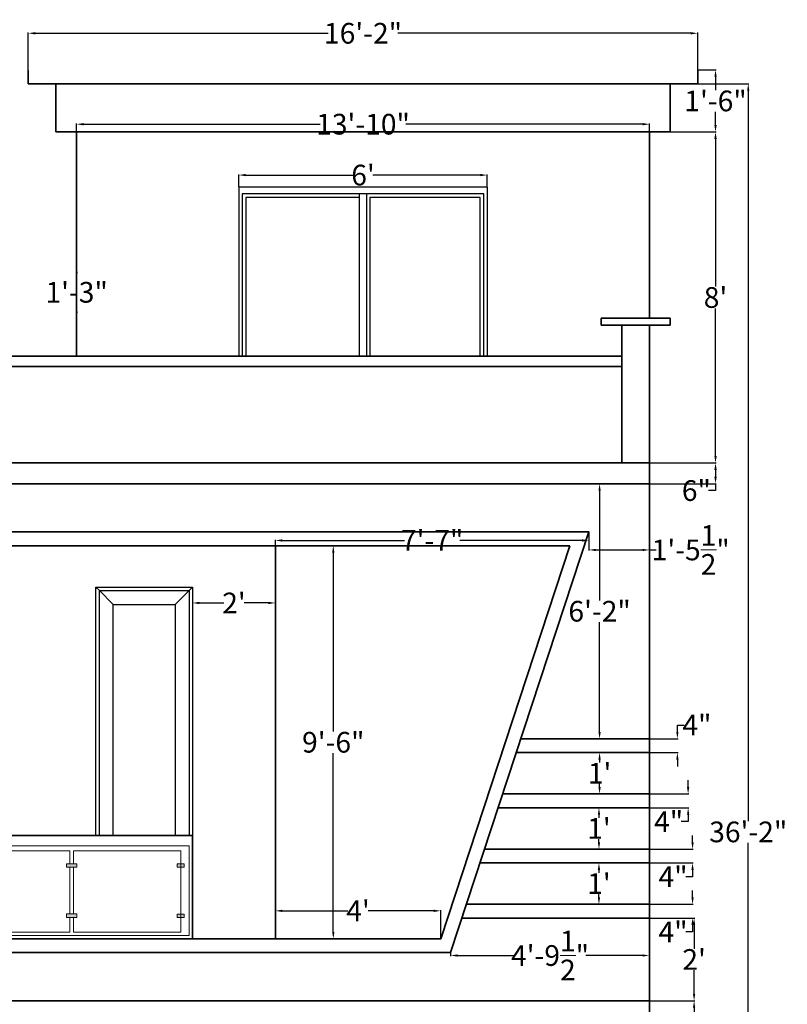
# Model space of a CAD drawing. Units: inches. Extents: x 786 to 1239, y 110 to 563.
# Tile 3 of 3: x 1017 to 1239, y 277 to 563. Entities that reach past the tile are written whole.
import ezdxf

# ---------------------------------------------------------------- set-up
doc = ezdxf.new("R2010")
doc.units = ezdxf.units.IN
doc.header["$MEASUREMENT"] = 0
for name, color, linetype, lineweight in [('A-ANNO-DIMS', 2, 'Continuous', 18), ('A-ELEV', 7, 'Continuous', 35), ('A-ELEV-PATT', 8, 'Continuous', 13), ('A-ELEV-RAIL', 3, 'Continuous', 18), ('A-GLAZ', 4, 'Continuous', 25)]:
    doc.layers.add(name, color=color, linetype=linetype, lineweight=lineweight)
doc.styles.get("Standard").update_dxf_attribs({"font": 'arial.ttf'})
doc.dimstyles.get("Standard").update_dxf_attribs({"dimtxt": 6, "dimasz": 2, "dimexe": 0.18, "dimexo": 0.0625, "dimgap": 0.09, "dimtad": 0, "dimtih": 1, "dimtoh": 1, "dimdec": 1, "dimzin": 0, "dimdsep": 46, "dimlunit": 4, "dimtxsty": 'Standard', "dimcen": 0.09, "dimadec": 0, "dimazin": 0, "dimtfac": 1, "dimtdec": 1, "dimtofl": 0, "dimtmove": 0, "dimatfit": 3, "dimfxl": 1, "dimtolj": 1, "dimtzin": 0, "dimarcsym": 0})

# ---------------------------------------------------------------- blocks, each defined once
blk = doc.blocks.new('*D10')
at = {"layer": 'A-ANNO-DIMS', "color": 0, "lineweight": -2, "transparency": 16777216}
for p, q in [((1199.19, 428.05), (1199.19, 408.71)), ((1181.65, 414.05), (1181.65, 408.71)), ((1183.65, 408.89), (1197.19, 408.89)), ((1199.19, 408.89), (1201.19, 408.89))]:
    blk.add_line(p, q, dxfattribs=at)
at = {"layer": 'A-ANNO-DIMS', "color": 0, "transparency": 16777216}
for points in [[(1183.65, 409.22), (1183.65, 408.56), (1181.65, 408.89)], [(1197.19, 409.22), (1197.19, 408.56), (1199.19, 408.89)]]:
    blk.add_solid(points, dxfattribs=at)
at = {"layer": 'Defpoints', "color": 0, "transparency": 16777216}
for p in [(1199.19, 428.11), (1181.65, 414.11), (1199.19, 408.89)]:
    blk.add_point(p, dxfattribs=at)
at = {"layer": 'A-ANNO-DIMS', "color": 0, "transparency": 16777216, "insert": (1211.16, 408.89), "char_height": 6, "attachment_point": 5}
blk.add_mtext('\\A1;1\'-5{\\H1x;\\S1/2;}"', dxfattribs=at)
blk = doc.blocks.new('*D11')
at = {"layer": 'A-ANNO-DIMS', "color": 0, "lineweight": -2, "transparency": 16777216}
for p, q in [((1090.86, 410.11), (1107.75, 410.11)), ((1107.57, 408.11), (1107.57, 356.26)), ((1107.57, 298.11), (1107.57, 349.96)), ((1090.86, 296.11), (1107.75, 296.11))]:
    blk.add_line(p, q, dxfattribs=at)
at = {"layer": 'A-ANNO-DIMS', "color": 0, "transparency": 16777216}
for points in [[(1107.24, 408.11), (1107.91, 408.11), (1107.57, 410.11)], [(1107.24, 298.11), (1107.91, 298.11), (1107.57, 296.11)]]:
    blk.add_solid(points, dxfattribs=at)
at = {"layer": 'Defpoints', "color": 0, "transparency": 16777216}
for p in [(1090.79, 410.11), (1107.57, 410.11), (1090.79, 296.11)]:
    blk.add_point(p, dxfattribs=at)
at = {"layer": 'A-ANNO-DIMS', "color": 0, "transparency": 16777216, "insert": (1107.57, 353.11), "char_height": 6, "attachment_point": 5}
blk.add_mtext('\\A1;9\'-6"', dxfattribs=at)
blk = doc.blocks.new('*D14')
at = {"layer": 'A-ANNO-DIMS', "color": 0, "lineweight": -2, "transparency": 16777216}
for p, q in [((1033.19, 489.11), (1033.19, 486.76)), ((1033.26, 491.11), (1033.37, 491.11)), ((1033.19, 478.11), (1033.19, 480.45)), ((1033.26, 476.11), (1033.37, 476.11))]:
    blk.add_line(p, q, dxfattribs=at)
at = {"layer": 'A-ANNO-DIMS', "color": 0, "transparency": 16777216}
for points in [[(1032.86, 489.11), (1033.53, 489.11), (1033.19, 491.11)], [(1032.86, 478.11), (1033.53, 478.11), (1033.19, 476.11)]]:
    blk.add_solid(points, dxfattribs=at)
at = {"layer": 'Defpoints', "color": 0, "transparency": 16777216}
for p in [(1033.19, 491.11), (1033.19, 491.11), (1033.19, 476.11)]:
    blk.add_point(p, dxfattribs=at)
at = {"layer": 'A-ANNO-DIMS', "color": 0, "transparency": 16777216, "insert": (1033.19, 483.61), "char_height": 6, "attachment_point": 5}
blk.add_mtext('\\A1;1\'-3"', dxfattribs=at)
blk = doc.blocks.new('*D15')
at = {"layer": 'A-ANNO-DIMS', "color": 0, "lineweight": -2, "transparency": 16777216}
for p, q in [((1080.19, 514.19), (1080.19, 517.79)), ((1082.19, 517.61), (1113.33, 517.61)), ((1150.19, 517.61), (1119.06, 517.61)), ((1152.19, 514.19), (1152.19, 517.79))]:
    blk.add_line(p, q, dxfattribs=at)
at = {"layer": 'A-ANNO-DIMS', "color": 0, "transparency": 16777216}
for points in [[(1082.19, 517.95), (1082.19, 517.28), (1080.19, 517.61)], [(1150.19, 517.95), (1150.19, 517.28), (1152.19, 517.61)]]:
    blk.add_solid(points, dxfattribs=at)
at = {"layer": 'Defpoints', "color": 0, "transparency": 16777216}
for p in [(1080.19, 517.61), (1080.19, 514.13), (1152.19, 514.13)]:
    blk.add_point(p, dxfattribs=at)
at = {"layer": 'A-ANNO-DIMS', "color": 0, "transparency": 16777216, "insert": (1116.19, 517.61), "char_height": 6, "attachment_point": 5}
blk.add_mtext("\\A1;6'", dxfattribs=at)
blk = doc.blocks.new('*D16')
at = {"layer": 'A-ANNO-DIMS', "color": 0, "lineweight": -2, "transparency": 16777216}
for p, q in [((1213.26, 548.11), (1218.53, 548.11)), ((1218.35, 546.11), (1218.35, 542.26)), ((1218.35, 532.11), (1218.35, 535.96)), ((1205.26, 530.11), (1218.53, 530.11))]:
    blk.add_line(p, q, dxfattribs=at)
at = {"layer": 'A-ANNO-DIMS', "color": 0, "transparency": 16777216}
for points in [[(1218.02, 546.11), (1218.69, 546.11), (1218.35, 548.11)], [(1218.02, 532.11), (1218.69, 532.11), (1218.35, 530.11)]]:
    blk.add_solid(points, dxfattribs=at)
at = {"layer": 'Defpoints', "color": 0, "transparency": 16777216}
for p in [(1213.19, 548.11), (1218.35, 548.11), (1205.19, 530.11)]:
    blk.add_point(p, dxfattribs=at)
at = {"layer": 'A-ANNO-DIMS', "color": 0, "transparency": 16777216, "insert": (1218.35, 539.11), "char_height": 6, "attachment_point": 5}
blk.add_mtext('\\A1;1\'-6"', dxfattribs=at)
blk = doc.blocks.new('*D17')
at = {"layer": 'A-ANNO-DIMS', "color": 0, "lineweight": -2, "transparency": 16777216}
for p, q in [((1019.19, 544.17), (1019.19, 558.92)), ((1021.19, 558.74), (1106.08, 558.74)), ((1211.19, 558.74), (1126.31, 558.74)), ((1213.19, 544.17), (1213.19, 558.92))]:
    blk.add_line(p, q, dxfattribs=at)
at = {"layer": 'A-ANNO-DIMS', "color": 0, "transparency": 16777216}
for points in [[(1021.19, 559.07), (1021.19, 558.41), (1019.19, 558.74)], [(1211.19, 559.07), (1211.19, 558.41), (1213.19, 558.74)]]:
    blk.add_solid(points, dxfattribs=at)
at = {"layer": 'Defpoints', "color": 0, "transparency": 16777216}
for p in [(1019.19, 558.74), (1019.19, 544.11), (1213.19, 544.11)]:
    blk.add_point(p, dxfattribs=at)
at = {"layer": 'A-ANNO-DIMS', "color": 0, "transparency": 16777216, "insert": (1116.19, 558.74), "char_height": 6, "attachment_point": 5}
blk.add_mtext('\\A1;16\'-2"', dxfattribs=at)
blk = doc.blocks.new('*D18')
at = {"layer": 'A-ANNO-DIMS', "color": 0, "lineweight": -2, "transparency": 16777216}
for p, q in [((1033.19, 530.17), (1033.19, 532.55)), ((1035.19, 532.37), (1103.75, 532.37)), ((1197.19, 532.37), (1128.64, 532.37)), ((1199.19, 530.17), (1199.19, 532.55))]:
    blk.add_line(p, q, dxfattribs=at)
at = {"layer": 'A-ANNO-DIMS', "color": 0, "transparency": 16777216}
for points in [[(1035.19, 532.7), (1035.19, 532.03), (1033.19, 532.37)], [(1197.19, 532.7), (1197.19, 532.03), (1199.19, 532.37)]]:
    blk.add_solid(points, dxfattribs=at)
at = {"layer": 'Defpoints', "color": 0, "transparency": 16777216}
for p in [(1199.19, 532.37), (1033.19, 530.11), (1199.19, 530.11)]:
    blk.add_point(p, dxfattribs=at)
at = {"layer": 'A-ANNO-DIMS', "color": 0, "transparency": 16777216, "insert": (1116.19, 532.37), "char_height": 6, "attachment_point": 5}
blk.add_mtext('\\A1;13\'-10"', dxfattribs=at)
blk = doc.blocks.new('*D19')
at = {"layer": 'A-ANNO-DIMS', "color": 0, "lineweight": -2, "transparency": 16777216}
for p, q in [((1207.3, 356.11), (1207.3, 358.11)), ((1207.3, 358.11), (1209.3, 358.11)), ((1199.26, 354.11), (1207.48, 354.11)), ((1199.26, 350.11), (1207.48, 350.11)), ((1207.3, 348.11), (1207.3, 346.11))]:
    blk.add_line(p, q, dxfattribs=at)
at = {"layer": 'A-ANNO-DIMS', "color": 0, "transparency": 16777216}
for points in [[(1206.97, 356.11), (1207.63, 356.11), (1207.3, 354.11)], [(1206.97, 348.11), (1207.63, 348.11), (1207.3, 350.11)]]:
    blk.add_solid(points, dxfattribs=at)
at = {"layer": 'Defpoints', "color": 0, "transparency": 16777216}
for p in [(1199.19, 354.11), (1207.3, 354.11), (1199.19, 350.11)]:
    blk.add_point(p, dxfattribs=at)
at = {"layer": 'A-ANNO-DIMS', "color": 0, "transparency": 16777216, "insert": (1212.96, 358.11), "char_height": 6, "attachment_point": 5}
blk.add_mtext('\\A1;4"', dxfattribs=at)
blk = doc.blocks.new('*D20')
at = {"layer": 'A-ANNO-DIMS', "color": 0, "lineweight": -2, "transparency": 16777216}
for p, q in [((1210.41, 340.11), (1210.41, 342.11)), ((1199.26, 338.11), (1210.59, 338.11)), ((1199.26, 334.11), (1210.59, 334.11)), ((1210.41, 332.11), (1210.41, 330.11)), ((1210.41, 330.11), (1208.41, 330.11))]:
    blk.add_line(p, q, dxfattribs=at)
at = {"layer": 'A-ANNO-DIMS', "color": 0, "transparency": 16777216}
for points in [[(1210.08, 340.11), (1210.75, 340.11), (1210.41, 338.11)], [(1210.08, 332.11), (1210.75, 332.11), (1210.41, 334.11)]]:
    blk.add_solid(points, dxfattribs=at)
at = {"layer": 'Defpoints', "color": 0, "transparency": 16777216}
for p in [(1199.19, 338.11), (1199.19, 334.11), (1210.41, 334.11)]:
    blk.add_point(p, dxfattribs=at)
at = {"layer": 'A-ANNO-DIMS', "color": 0, "transparency": 16777216, "insert": (1204.76, 330.11), "char_height": 6, "attachment_point": 5}
blk.add_mtext('\\A1;4"', dxfattribs=at)
blk = doc.blocks.new('*D21')
at = {"layer": 'A-ANNO-DIMS', "color": 0, "lineweight": -2, "transparency": 16777216}
for p, q in [((1211.7, 324.11), (1211.7, 326.11)), ((1199.26, 322.11), (1211.88, 322.11)), ((1199.26, 318.11), (1211.88, 318.11)), ((1211.7, 316.11), (1211.7, 314.11)), ((1211.7, 314.11), (1209.7, 314.11))]:
    blk.add_line(p, q, dxfattribs=at)
at = {"layer": 'A-ANNO-DIMS', "color": 0, "transparency": 16777216}
for points in [[(1211.37, 324.11), (1212.03, 324.11), (1211.7, 322.11)], [(1211.37, 316.11), (1212.03, 316.11), (1211.7, 318.11)]]:
    blk.add_solid(points, dxfattribs=at)
at = {"layer": 'Defpoints', "color": 0, "transparency": 16777216}
for p in [(1199.19, 322.11), (1199.19, 318.11), (1211.7, 318.11)]:
    blk.add_point(p, dxfattribs=at)
at = {"layer": 'A-ANNO-DIMS', "color": 0, "transparency": 16777216, "insert": (1206.04, 314.11), "char_height": 6, "attachment_point": 5}
blk.add_mtext('\\A1;4"', dxfattribs=at)
blk = doc.blocks.new('*D22')
at = {"layer": 'A-ANNO-DIMS', "color": 0, "lineweight": -2, "transparency": 16777216}
for p, q in [((1211.7, 308.11), (1211.7, 310.11)), ((1199.26, 306.11), (1211.88, 306.11)), ((1199.26, 302.11), (1211.88, 302.11)), ((1211.7, 300.11), (1211.7, 298.11)), ((1211.7, 298.11), (1209.7, 298.11))]:
    blk.add_line(p, q, dxfattribs=at)
at = {"layer": 'A-ANNO-DIMS', "color": 0, "transparency": 16777216}
for points in [[(1211.37, 308.11), (1212.03, 308.11), (1211.7, 306.11)], [(1211.37, 300.11), (1212.03, 300.11), (1211.7, 302.11)]]:
    blk.add_solid(points, dxfattribs=at)
at = {"layer": 'Defpoints', "color": 0, "transparency": 16777216}
for p in [(1199.19, 306.11), (1199.19, 302.11), (1211.7, 302.11)]:
    blk.add_point(p, dxfattribs=at)
at = {"layer": 'A-ANNO-DIMS', "color": 0, "transparency": 16777216, "insert": (1206.04, 298.11), "char_height": 6, "attachment_point": 5}
blk.add_mtext('\\A1;4"', dxfattribs=at)
blk = doc.blocks.new('*D23')
at = {"layer": 'A-ANNO-DIMS', "color": 0, "lineweight": -2, "transparency": 16777216}
for p, q in [((1199.13, 350.11), (1184.57, 350.11)), ((1184.75, 348.11), (1184.75, 347.21)), ((1184.75, 340.11), (1184.75, 341.01)), ((1199.13, 338.11), (1184.57, 338.11))]:
    blk.add_line(p, q, dxfattribs=at)
at = {"layer": 'A-ANNO-DIMS', "color": 0, "transparency": 16777216}
for points in [[(1184.42, 348.11), (1185.08, 348.11), (1184.75, 350.11)], [(1184.42, 340.11), (1185.08, 340.11), (1184.75, 338.11)]]:
    blk.add_solid(points, dxfattribs=at)
at = {"layer": 'Defpoints', "color": 0, "transparency": 16777216}
for p in [(1199.19, 350.11), (1184.75, 338.11), (1199.19, 338.11)]:
    blk.add_point(p, dxfattribs=at)
at = {"layer": 'A-ANNO-DIMS', "color": 0, "transparency": 16777216, "insert": (1184.75, 344.11), "char_height": 6, "attachment_point": 5}
blk.add_mtext("\\A1;1'", dxfattribs=at)
blk = doc.blocks.new('*D36')
at = {"layer": 'A-ANNO-DIMS', "color": 0, "lineweight": -2, "transparency": 16777216}
for p, q in [((1199.26, 278.11), (1212.32, 278.11)), ((1212.14, 276.11), (1212.14, 274.11)), ((1199.26, 272.11), (1212.32, 272.11)), ((1212.14, 272.11), (1212.14, 270.11)), ((1212.14, 270.11), (1210.14, 270.11))]:
    blk.add_line(p, q, dxfattribs=at)
at = {"layer": 'A-ANNO-DIMS', "color": 0, "transparency": 16777216}
for points in [[(1211.81, 276.11), (1212.47, 276.11), (1212.14, 278.11)], [(1211.81, 274.11), (1212.47, 274.11), (1212.14, 272.11)]]:
    blk.add_solid(points, dxfattribs=at)
at = {"layer": 'Defpoints', "color": 0, "transparency": 16777216}
for p in [(1199.19, 278.11), (1199.19, 272.11), (1212.14, 272.11)]:
    blk.add_point(p, dxfattribs=at)
at = {"layer": 'A-ANNO-DIMS', "color": 0, "transparency": 16777216, "insert": (1206.58, 270.11), "char_height": 6, "attachment_point": 5}
blk.add_mtext('\\A1;6"', dxfattribs=at)
blk = doc.blocks.new('*D37')
at = {"layer": 'A-ANNO-DIMS', "color": 0, "lineweight": -2, "transparency": 16777216}
for p, q in [((1199.26, 302.11), (1212.32, 302.11)), ((1212.14, 300.11), (1212.14, 293.21)), ((1212.14, 280.11), (1212.14, 287.01)), ((1199.26, 278.11), (1212.32, 278.11))]:
    blk.add_line(p, q, dxfattribs=at)
at = {"layer": 'A-ANNO-DIMS', "color": 0, "transparency": 16777216}
for points in [[(1211.81, 300.11), (1212.47, 300.11), (1212.14, 302.11)], [(1211.81, 280.11), (1212.47, 280.11), (1212.14, 278.11)]]:
    blk.add_solid(points, dxfattribs=at)
at = {"layer": 'Defpoints', "color": 0, "transparency": 16777216}
for p in [(1199.19, 302.11), (1212.14, 302.11), (1199.19, 278.11)]:
    blk.add_point(p, dxfattribs=at)
at = {"layer": 'A-ANNO-DIMS', "color": 0, "transparency": 16777216, "insert": (1212.14, 290.11), "char_height": 6, "attachment_point": 5}
blk.add_mtext("\\A1;2'", dxfattribs=at)
blk = doc.blocks.new('*D38')
at = {"layer": 'A-ANNO-DIMS', "color": 0, "lineweight": -2, "transparency": 16777216}
for p, q in [((1141.59, 292.05), (1141.59, 291.08)), ((1199.19, 278.17), (1199.19, 291.44)), ((1143.59, 291.26), (1160.02, 291.26)), ((1197.19, 291.26), (1180.77, 291.26))]:
    blk.add_line(p, q, dxfattribs=at)
at = {"layer": 'A-ANNO-DIMS', "color": 0, "transparency": 16777216}
for points in [[(1143.59, 291.59), (1143.59, 290.93), (1141.59, 291.26)], [(1197.19, 291.59), (1197.19, 290.93), (1199.19, 291.26)]]:
    blk.add_solid(points, dxfattribs=at)
at = {"layer": 'Defpoints', "color": 0, "transparency": 16777216}
for p in [(1141.59, 292.11), (1199.19, 291.26), (1199.19, 278.11)]:
    blk.add_point(p, dxfattribs=at)
at = {"layer": 'A-ANNO-DIMS', "color": 0, "transparency": 16777216, "insert": (1170.39, 291.26), "char_height": 6, "attachment_point": 5}
blk.add_mtext('\\A1;4\'-9{\\H1x;\\S1/2;}"', dxfattribs=at)
blk = doc.blocks.new('*D39')
at = {"layer": 'A-ANNO-DIMS', "color": 0, "lineweight": -2, "transparency": 16777216}
for p, q in [((1199.26, 530.11), (1218.53, 530.11)), ((1218.35, 528.11), (1218.35, 485.26)), ((1218.35, 436.11), (1218.35, 478.96)), ((1199.26, 434.11), (1218.53, 434.11))]:
    blk.add_line(p, q, dxfattribs=at)
at = {"layer": 'A-ANNO-DIMS', "color": 0, "transparency": 16777216}
for points in [[(1218.02, 528.11), (1218.69, 528.11), (1218.35, 530.11)], [(1218.02, 436.11), (1218.69, 436.11), (1218.35, 434.11)]]:
    blk.add_solid(points, dxfattribs=at)
at = {"layer": 'Defpoints', "color": 0, "transparency": 16777216}
for p in [(1199.19, 530.11), (1218.35, 530.11), (1199.19, 434.11)]:
    blk.add_point(p, dxfattribs=at)
at = {"layer": 'A-ANNO-DIMS', "color": 0, "transparency": 16777216, "insert": (1218.35, 482.11), "char_height": 6, "attachment_point": 5}
blk.add_mtext("\\A1;8'", dxfattribs=at)
blk = doc.blocks.new('*D40')
at = {"layer": 'A-ANNO-DIMS', "color": 0, "lineweight": -2, "transparency": 16777216}
for p, q in [((1199.26, 434.11), (1218.53, 434.11)), ((1218.35, 432.11), (1218.35, 430.11)), ((1199.26, 428.11), (1218.53, 428.11)), ((1218.35, 426.11), (1216.35, 426.11)), ((1218.35, 428.11), (1218.35, 426.11))]:
    blk.add_line(p, q, dxfattribs=at)
at = {"layer": 'A-ANNO-DIMS', "color": 0, "transparency": 16777216}
for points in [[(1218.02, 432.11), (1218.69, 432.11), (1218.35, 434.11)], [(1218.02, 430.11), (1218.69, 430.11), (1218.35, 428.11)]]:
    blk.add_solid(points, dxfattribs=at)
at = {"layer": 'Defpoints', "color": 0, "transparency": 16777216}
for p in [(1199.19, 434.11), (1199.19, 428.11), (1218.35, 428.11)]:
    blk.add_point(p, dxfattribs=at)
at = {"layer": 'A-ANNO-DIMS', "color": 0, "transparency": 16777216, "insert": (1212.8, 426.11), "char_height": 6, "attachment_point": 5}
blk.add_mtext('\\A1;6"', dxfattribs=at)
blk = doc.blocks.new('*D48')
at = {"layer": 'A-ANNO-DIMS', "color": 0, "lineweight": -2, "transparency": 16777216}
for p, q in [((1205.26, 544.11), (1228.02, 544.11)), ((1227.84, 542.11), (1227.84, 330.26)), ((1227.84, 112.11), (1227.84, 323.95)), ((1199.26, 110.11), (1228.02, 110.11))]:
    blk.add_line(p, q, dxfattribs=at)
at = {"layer": 'A-ANNO-DIMS', "color": 0, "transparency": 16777216}
for points in [[(1227.51, 542.11), (1228.17, 542.11), (1227.84, 544.11)], [(1227.51, 112.11), (1228.17, 112.11), (1227.84, 110.11)]]:
    blk.add_solid(points, dxfattribs=at)
at = {"layer": 'Defpoints', "color": 0, "transparency": 16777216}
for p in [(1205.19, 544.11), (1199.19, 110.11), (1227.84, 110.11)]:
    blk.add_point(p, dxfattribs=at)
at = {"layer": 'A-ANNO-DIMS', "color": 0, "transparency": 16777216, "insert": (1227.84, 327.11), "char_height": 6, "attachment_point": 5}
blk.add_mtext('\\A1;36\'-2"', dxfattribs=at)
blk = doc.blocks.new('*D49')
at = {"layer": 'A-ANNO-DIMS', "color": 0, "lineweight": -2, "transparency": 16777216}
for p, q in [((1090.79, 410.17), (1090.79, 411.83)), ((1092.79, 411.65), (1128.18, 411.65)), ((1179.65, 411.65), (1144.26, 411.65)), ((1181.65, 414.05), (1181.65, 411.47))]:
    blk.add_line(p, q, dxfattribs=at)
at = {"layer": 'A-ANNO-DIMS', "color": 0, "transparency": 16777216}
for points in [[(1092.79, 411.98), (1092.79, 411.31), (1090.79, 411.65)], [(1179.65, 411.98), (1179.65, 411.31), (1181.65, 411.65)]]:
    blk.add_solid(points, dxfattribs=at)
at = {"layer": 'Defpoints', "color": 0, "transparency": 16777216}
for p in [(1181.65, 414.11), (1181.65, 411.65), (1090.79, 410.11)]:
    blk.add_point(p, dxfattribs=at)
at = {"layer": 'A-ANNO-DIMS', "color": 0, "transparency": 16777216, "insert": (1136.22, 411.65), "char_height": 6, "attachment_point": 5}
blk.add_mtext('\\A1;7\'-7"', dxfattribs=at)
blk = doc.blocks.new('*D50')
at = {"layer": 'A-ANNO-DIMS', "color": 0, "lineweight": -2, "transparency": 16777216}
for p, q in [((1090.79, 296.17), (1090.79, 304.4)), ((1092.79, 304.22), (1111.77, 304.22)), ((1136.7, 304.22), (1117.72, 304.22)), ((1138.7, 296.17), (1138.7, 304.4))]:
    blk.add_line(p, q, dxfattribs=at)
at = {"layer": 'A-ANNO-DIMS', "color": 0, "transparency": 16777216}
for points in [[(1092.79, 304.55), (1092.79, 303.89), (1090.79, 304.22)], [(1136.7, 304.55), (1136.7, 303.89), (1138.7, 304.22)]]:
    blk.add_solid(points, dxfattribs=at)
at = {"layer": 'Defpoints', "color": 0, "transparency": 16777216}
for p in [(1090.79, 304.22), (1090.79, 296.11), (1138.7, 296.11)]:
    blk.add_point(p, dxfattribs=at)
at = {"layer": 'A-ANNO-DIMS', "color": 0, "transparency": 16777216, "insert": (1114.74, 304.22), "char_height": 6, "attachment_point": 5}
blk.add_mtext("\\A1;4'", dxfattribs=at)
blk = doc.blocks.new('*D55')
at = {"layer": 'A-ANNO-DIMS', "color": 0, "lineweight": -2, "transparency": 16777216}
for p, q in [((1090.79, 410.05), (1090.79, 393.33)), ((1066.79, 398.05), (1066.79, 393.33)), ((1068.79, 393.51), (1075.89, 393.51)), ((1088.79, 393.51), (1081.7, 393.51))]:
    blk.add_line(p, q, dxfattribs=at)
at = {"layer": 'A-ANNO-DIMS', "color": 0, "transparency": 16777216}
for points in [[(1068.79, 393.84), (1068.79, 393.18), (1066.79, 393.51)], [(1088.79, 393.84), (1088.79, 393.18), (1090.79, 393.51)]]:
    blk.add_solid(points, dxfattribs=at)
at = {"layer": 'Defpoints', "color": 0, "transparency": 16777216}
for p in [(1090.79, 410.11), (1066.79, 398.11), (1066.79, 393.51)]:
    blk.add_point(p, dxfattribs=at)
at = {"layer": 'A-ANNO-DIMS', "color": 0, "transparency": 16777216, "insert": (1078.79, 393.51), "char_height": 6, "attachment_point": 5}
blk.add_mtext("\\A1;2'", dxfattribs=at)
blk = doc.blocks.new('*D56')
at = {"layer": 'A-ANNO-DIMS', "color": 0, "lineweight": -2, "transparency": 16777216}
for p, q in [((1199.13, 334.11), (1184.39, 334.11)), ((1184.57, 332.11), (1184.57, 331.21)), ((1184.57, 324.11), (1184.57, 325.01)), ((1199.13, 322.11), (1184.39, 322.11))]:
    blk.add_line(p, q, dxfattribs=at)
at = {"layer": 'A-ANNO-DIMS', "color": 0, "transparency": 16777216}
for points in [[(1184.24, 332.11), (1184.9, 332.11), (1184.57, 334.11)], [(1184.24, 324.11), (1184.9, 324.11), (1184.57, 322.11)]]:
    blk.add_solid(points, dxfattribs=at)
at = {"layer": 'Defpoints', "color": 0, "transparency": 16777216}
for p in [(1199.19, 334.11), (1184.57, 322.11), (1199.19, 322.11)]:
    blk.add_point(p, dxfattribs=at)
at = {"layer": 'A-ANNO-DIMS', "color": 0, "transparency": 16777216, "insert": (1184.57, 328.11), "char_height": 6, "attachment_point": 5}
blk.add_mtext("\\A1;1'", dxfattribs=at)
blk = doc.blocks.new('*D57')
at = {"layer": 'A-ANNO-DIMS', "color": 0, "lineweight": -2, "transparency": 16777216}
for p, q in [((1199.13, 318.11), (1184.39, 318.11)), ((1184.57, 316.11), (1184.57, 315.21)), ((1184.57, 308.11), (1184.57, 309.01)), ((1199.13, 306.11), (1184.39, 306.11))]:
    blk.add_line(p, q, dxfattribs=at)
at = {"layer": 'A-ANNO-DIMS', "color": 0, "transparency": 16777216}
for points in [[(1184.24, 316.11), (1184.9, 316.11), (1184.57, 318.11)], [(1184.24, 308.11), (1184.9, 308.11), (1184.57, 306.11)]]:
    blk.add_solid(points, dxfattribs=at)
at = {"layer": 'Defpoints', "color": 0, "transparency": 16777216}
for p in [(1199.19, 318.11), (1184.57, 306.11), (1199.19, 306.11)]:
    blk.add_point(p, dxfattribs=at)
at = {"layer": 'A-ANNO-DIMS', "color": 0, "transparency": 16777216, "insert": (1184.57, 312.11), "char_height": 6, "attachment_point": 5}
blk.add_mtext("\\A1;1'", dxfattribs=at)
blk = doc.blocks.new('*D58')
at = {"layer": 'A-ANNO-DIMS', "color": 0, "lineweight": -2, "transparency": 16777216}
for p, q in [((1199.13, 428.11), (1184.57, 428.11)), ((1184.75, 426.11), (1184.75, 394.26)), ((1184.75, 356.11), (1184.75, 387.96)), ((1199.13, 354.11), (1184.57, 354.11))]:
    blk.add_line(p, q, dxfattribs=at)
at = {"layer": 'A-ANNO-DIMS', "color": 0, "transparency": 16777216}
for points in [[(1184.42, 426.11), (1185.08, 426.11), (1184.75, 428.11)], [(1184.42, 356.11), (1185.08, 356.11), (1184.75, 354.11)]]:
    blk.add_solid(points, dxfattribs=at)
at = {"layer": 'Defpoints', "color": 0, "transparency": 16777216}
for p in [(1184.75, 428.11), (1199.19, 428.11), (1199.19, 354.11)]:
    blk.add_point(p, dxfattribs=at)
at = {"layer": 'A-ANNO-DIMS', "color": 0, "transparency": 16777216, "insert": (1184.75, 391.11), "char_height": 6, "attachment_point": 5}
blk.add_mtext('\\A1;6\'-2"', dxfattribs=at)
blk = doc.blocks.new('GLASS-CLAMP-A')
for p, q in [((0, 1), (3, 1)), ((0, 1), (0, 0)), ((3, 0), (3, 1)), ((3, 0), (0, 0))]:
    blk.add_line(p, q)
blk = doc.blocks.new('GLASS-CLAMP-B')
for p, q in [((0, 1), (2, 1)), ((0, 0), (0, 1)), ((2, 0), (2, 1)), ((0, 0), (2, 0))]:
    blk.add_line(p, q)

msp = doc.modelspace()

# ---------------------------------------------------------------- hatches: boundary and pattern name
at = {"layer": 'A-ELEV-PATT'}
h = msp.add_hatch(color=256, dxfattribs=at)
h.dxf.hatch_style = 1
h.paths.add_polyline_path([(842.59, 317.86), (841.59, 317.86), (841.59, 316.86), (842.59, 316.86)])
h.paths.add_polyline_path([(841.59, 317.86), (840.59, 317.86), (840.59, 316.86), (841.59, 316.86)])
h.paths.add_polyline_path([(842.59, 303.29), (841.59, 303.29), (841.59, 302.31), (842.59, 302.31)])
h.paths.add_polyline_path([(841.59, 303.29), (840.59, 303.29), (840.59, 302.31), (841.59, 302.31)])
h.paths.add_polyline_path([(1064.36, 317.86), (1063.36, 317.86), (1063.36, 316.86), (1064.36, 316.86)])
h.paths.add_polyline_path([(1063.36, 317.86), (1062.36, 317.86), (1062.36, 316.86), (1063.36, 316.86)])
h.paths.add_polyline_path([(1064.36, 303.29), (1063.36, 303.29), (1063.36, 302.31), (1064.36, 302.31)])
h.paths.add_polyline_path([(1063.36, 303.29), (1062.36, 303.29), (1062.36, 302.31), (1063.36, 302.31)])
h = msp.add_hatch(color=256, dxfattribs=at)
h.dxf.hatch_style = 1
h.paths.add_polyline_path([(874.65, 317.86), (871.65, 317.86), (871.65, 316.86), (874.65, 316.86)])
h.paths.add_polyline_path([(906.56, 317.86), (903.56, 317.86), (903.56, 316.86), (906.56, 316.86)])
h.paths.add_polyline_path([(938.2, 317.86), (935.2, 317.86), (935.2, 316.86), (938.2, 316.86)])
h.paths.add_polyline_path([(969.78, 317.86), (966.78, 317.86), (966.78, 316.86), (969.78, 316.86)])
h.paths.add_polyline_path([(1001.46, 317.86), (998.46, 317.86), (998.46, 316.86), (1001.46, 316.86)])
h.paths.add_polyline_path([(1033.24, 317.86), (1030.24, 317.86), (1030.24, 316.86), (1033.24, 316.86)])
h.paths.add_polyline_path([(1033.24, 303.31), (1030.24, 303.31), (1030.24, 302.31), (1033.24, 302.31)])
h.paths.add_polyline_path([(1001.46, 303.31), (998.46, 303.31), (998.46, 302.31), (1001.46, 302.31)])
h.paths.add_polyline_path([(969.78, 303.31), (966.78, 303.31), (966.78, 302.31), (969.78, 302.31)])
h.paths.add_polyline_path([(938.2, 303.31), (935.2, 303.31), (935.2, 302.31), (938.2, 302.31)])
h.paths.add_polyline_path([(906.56, 303.31), (903.56, 303.31), (903.56, 302.31), (906.56, 302.31)])
h.paths.add_polyline_path([(874.65, 303.31), (871.65, 303.31), (871.65, 302.31), (874.65, 302.31)])

# ---------------------------------------------------------------- linework, layer by layer
at = {"layer": 'A-ELEV'}
for p, q in [((1019.19, 547.93), (1019.19, 544.11)), ((1213.19, 544.11), (1213.19, 548.11)), ((1213.19, 544.11), (1019.19, 544.11)), ((1027.19, 530.11), (1027.19, 544.11)), ((1205.19, 530.11), (1205.19, 544.11)), ((1205.19, 530.11), (1027.19, 530.11)), ((1033.19, 465.11), (1033.19, 530.11)), ((1199.19, 530.11), (1199.19, 476.11)), ((1205.19, 476.11), (1185.19, 476.11)), ((1185.19, 474.11), (1185.19, 476.11)), ((1199.19, 474.11), (1185.19, 474.11)), ((1191.19, 434.11), (1191.19, 474.11)), ((1199.19, 434.11), (1199.19, 474.11)), ((1199.19, 474.11), (1205.19, 474.11)), ((1205.19, 474.11), (1205.19, 476.11)), ((1191.19, 465.11), (983.67, 465.11)), ((1191.19, 462.11), (983.67, 462.11)), ((1191.19, 434.11), (815.19, 434.11)), ((1199.19, 434.11), (1191.19, 434.11)), ((1199.19, 428.11), (1199.19, 434.11)), ((1199.19, 428.11), (815.19, 428.11)), ((1199.19, 410.11), (1199.19, 428.11)), ((1176.13, 410.11), (839.19, 410.11)), ((1090.79, 296.11), (1090.79, 410.11)), ((1176.13, 410.11), (1138.7, 296.11)), ((1199.19, 278.11), (1199.19, 410.11)), ((1199.19, 354.11), (1161.95, 354.11)), ((1160.64, 350.11), (1199.19, 350.11)), ((1199.19, 338.11), (1156.7, 338.11)), ((1155.38, 334.11), (1199.19, 334.11)), ((1066.79, 326.11), (839.19, 326.11)), ((1066.79, 326.11), (1066.79, 296.11)), ((1199.19, 322.11), (1151.44, 322.11)), ((1150.13, 318.11), (1199.19, 318.11)), ((1199.19, 306.11), (1146.19, 306.11)), ((1144.88, 302.11), (1199.19, 302.11)), ((1138.7, 296.11), (839.19, 296.11)), ((1199.19, 278.11), (815.19, 278.11)), ((1199.19, 272.11), (1199.19, 278.11))]:
    msp.add_line(p, q, dxfattribs=at)
msp.add_lwpolyline([(1141.59, 292.11), (835.19, 292.11), (835.19, 414.11), (1181.65, 414.11)], close=True, dxfattribs=at)
at = {"layer": 'A-ELEV-RAIL'}
for p, q in [((1065.79, 323.11), (840.19, 323.11)), ((1065.79, 297.11), (1065.79, 323.11)), ((1065.79, 297.11), (840.19, 297.11))]:
    msp.add_line(p, q, dxfattribs=at)
for points in [[(1000.18, 317.86), (1000.18, 321.66), (1031.24, 321.66), (1031.24, 317.86)], [(1032.31, 317.86), (1032.31, 321.66), (1063.36, 321.66), (1063.36, 298.05), (1032.31, 298.05), (1032.31, 302.31)], [(1031.24, 316.86), (1031.24, 303.31)], [(1032.31, 303.31), (1032.31, 316.86)], [(1031.24, 302.31), (1031.24, 298.05), (1000.18, 298.05), (1000.18, 302.31)]]:
    msp.add_lwpolyline(points, dxfattribs=at)
at = {"layer": 'A-GLAZ'}
for p, q in [((1080.19, 514.13), (1080.19, 465.11)), ((1152.19, 514.13), (1080.19, 514.13)), ((1152.19, 514.13), (1152.19, 465.11)), ((1115.19, 465.11), (1115.19, 512.13)), ((1117.19, 512.13), (1117.19, 465.11)), ((1118.19, 511.13), (1118.19, 465.11)), ((1039.79, 397.11), (1038.79, 398.11)), ((1043.79, 393.11), (1039.79, 397.11)), ((1061.79, 393.11), (1065.79, 397.11)), ((1065.79, 397.11), (1066.79, 398.11))]:
    msp.add_line(p, q, dxfattribs=at)
for points in [[(1151.19, 465.11), (1151.19, 512.13), (1081.19, 512.13), (1081.19, 465.11)], [(1115.19, 511.13), (1082.19, 511.13), (1082.19, 465.11)], [(1150.19, 465.11), (1150.19, 511.13), (1118.19, 511.13)], [(1038.79, 326.11), (1038.79, 398.11), (1066.79, 398.11), (1066.79, 326.11)], [(1039.79, 326.11), (1039.79, 397.11), (1065.79, 397.11), (1065.79, 326.11)], [(1043.79, 326.11), (1043.79, 393.11), (1061.79, 393.11), (1061.79, 326.11)]]:
    msp.add_lwpolyline(points, dxfattribs=at)

# ---------------------------------------------------------------- block references
at = {"layer": 'A-ELEV-RAIL'}
for name, p, rotation in [('GLASS-CLAMP-A', (1033.24, 317.86), 180), ('GLASS-CLAMP-B', (1064.36, 317.86), 180), ('GLASS-CLAMP-A', (1033.24, 303.31), 180), ('GLASS-CLAMP-B', (1062.36, 302.3), 359.7010863405159)]:
    msp.add_blockref(name, p, dxfattribs=dict(at, rotation=rotation))

# ---------------------------------------------------------------- dimensions: what is measured, and where the dimension line sits
at = {"layer": 'A-ANNO-DIMS'}
for base, p1, p2, picture, middle in [((1019.19, 558.74), (1213.19, 544.11), (1019.19, 544.11), '*D17', (1116.19, 558.74)), ((1199.19, 532.37), (1033.19, 530.11), (1199.19, 530.11), '*D18', (1116.19, 532.37)), ((1080.19, 517.61), (1152.19, 514.13), (1080.19, 514.13), '*D15', (1116.19, 517.61)), ((1199.19, 408.89), (1181.65, 414.11), (1199.19, 428.11), '*D10', (1211.16, 408.89)), ((1181.65, 411.65), (1090.79, 410.11), (1181.65, 414.11), '*D49', (1136.22, 411.65)), ((1066.79, 393.51), (1090.79, 410.11), (1066.79, 398.11), '*D55', (1078.79, 393.51)), ((1090.79, 304.22), (1138.7, 296.11), (1090.79, 296.11), '*D50', (1114.74, 304.22)), ((1199.19, 291.26), (1141.59, 292.11), (1199.19, 278.11), '*D38', (1170.39, 291.26))]:
    dim = msp.add_linear_dim(base=base, p1=p1, p2=p2, dimstyle='Standard', override={"dimclrd": 0, "dimclre": 0, "dimclrt": 0}, dxfattribs=at)
    dim.commit()
    dim.dimension.update_dxf_attribs({"geometry": picture, "text_midpoint": middle})
for base, p1, p2, picture, middle in [((1218.35, 548.11), (1205.19, 530.11), (1213.19, 548.11), '*D16', (1218.35, 539.11)), ((1227.84, 110.11), (1205.19, 544.11), (1199.19, 110.11), '*D48', (1227.84, 327.11)), ((1218.35, 530.11), (1199.19, 434.11), (1199.19, 530.11), '*D39', (1218.35, 482.11)), ((1033.19, 491.11), (1033.19, 476.11), (1033.19, 491.11), '*D14', (1033.19, 483.61)), ((1218.35, 428.11), (1199.19, 434.11), (1199.19, 428.11), '*D40', (1212.8, 426.11)), ((1184.75, 428.11), (1199.19, 354.11), (1199.19, 428.11), '*D58', (1184.75, 391.11)), ((1107.57, 410.11), (1090.79, 296.11), (1090.79, 410.11), '*D11', (1107.57, 353.11)), ((1207.3, 354.11), (1199.19, 350.11), (1199.19, 354.11), '*D19', (1212.96, 358.11)), ((1184.75, 338.11), (1199.19, 350.11), (1199.19, 338.11), '*D23', (1184.75, 344.11)), ((1210.41, 334.11), (1199.19, 338.11), (1199.19, 334.11), '*D20', (1204.76, 330.11)), ((1184.57, 322.11), (1199.19, 334.11), (1199.19, 322.11), '*D56', (1184.57, 328.11)), ((1211.7, 318.11), (1199.19, 322.11), (1199.19, 318.11), '*D21', (1206.04, 314.11)), ((1184.57, 306.11), (1199.19, 318.11), (1199.19, 306.11), '*D57', (1184.57, 312.11)), ((1211.7, 302.11), (1199.19, 306.11), (1199.19, 302.11), '*D22', (1206.04, 298.11)), ((1212.14, 302.11), (1199.19, 278.11), (1199.19, 302.11), '*D37', (1212.14, 290.11)), ((1212.14, 272.11), (1199.19, 278.11), (1199.19, 272.11), '*D36', (1206.58, 270.11))]:
    dim = msp.add_linear_dim(base=base, p1=p1, p2=p2, angle=90, dimstyle='Standard', override={"dimclrd": 0, "dimclre": 0, "dimclrt": 0}, dxfattribs=at)
    dim.commit()
    dim.dimension.update_dxf_attribs({"geometry": picture, "text_midpoint": middle})

doc.saveas('drawing.dxf')
